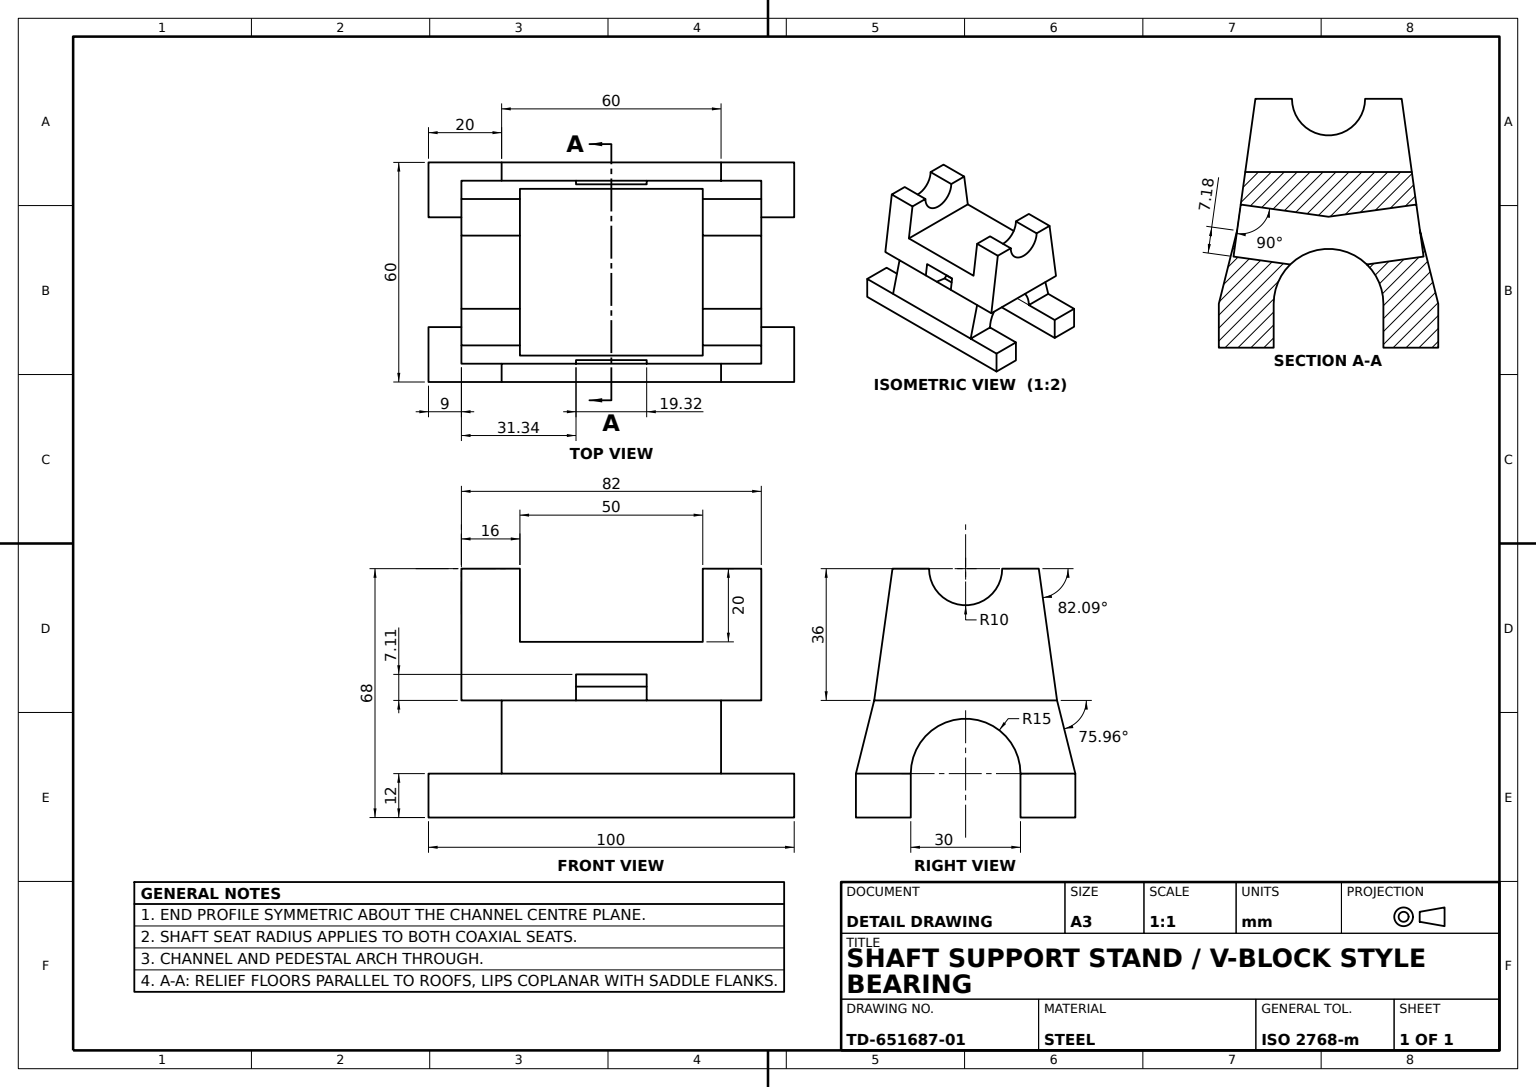
from build123d import *

# Parameters (mm, degrees)
BASE_BLOCK_DEPTH             = 12
BASE_CHANNEL_CUT_30X15_DEPTH = 73
TAPERED_PEDESTAL_DEPTH       = 60
SADDLE_BODY_DEPTH            = 82
SADDLE_RECESS_CUT_DEPTH      = 20
SIDE_RELIEF_SKETCH_W         = 19.32494716
SIDE_RELIEF_SKETCH_H         = 14.354217055
SIDE_RELIEF_CUT_DEPTH        = 28


with BuildPart() as part:
    # Base Profile Sketch → Base Block (new body)
    with BuildSketch(Plane(origin=(0, 0, 0), x_dir=(1, 0, 0), z_dir=(0, 1, 0))):
        Polygon((0, 0), (30, 0), (30, 100), (-30, 100), (-30, 0), align=None)
    extrude(amount=BASE_BLOCK_DEPTH)

    # Base Channel Sketch → Base Channel Cut 30x15 (cut)
    with BuildSketch(Plane(origin=(0, 12, 0), x_dir=(1, 0, 0), z_dir=(0, 1, 0))):
        Polygon((0, 0), (15, 0), (15, 100), (-15, 100), (-15, 0), align=None)
    extrude(amount=-BASE_CHANNEL_CUT_30X15_DEPTH, mode=Mode.SUBTRACT)


with BuildPart() as base_channel_cut_30x15_piece_1:
    # of the separate pieces the step leaves, piece 1, a body of its own (base_channel_cut_30x15_pieces)
    add(part.part.solids().sort_by_distance((30, 0, 0))[0])



with BuildPart() as base_channel_cut_30x15_piece_2:
    # of the separate pieces the step leaves, piece 2, a body of its own (base_channel_cut_30x15_pieces)
    add(part.part.solids().sort_by_distance((-15, 12, 0))[0])


with BuildPart() as base_channel_cut_30x15_piece_1_1:
    add(base_channel_cut_30x15_piece_1.part)

    add(base_channel_cut_30x15_piece_2.part)  # Tapered Pedestal merges Base Channel Cut 30x15 piece 2
    # Pedestal Profile Sketch → Tapered Pedestal (add)
    with BuildSketch(Plane.XY.offset(-20)):
        with BuildLine():
            Line((0, 32), (25, 32))
            Line((25, 32), (30, 12))
            Line((30, 12), (15, 12))
            ThreePointArc((15, 12), (0, 27), (-15, 12))
            Line((-15, 12), (-30, 12))
            Line((-30, 12), (-25, 32))
            Line((-25, 32), (0, 32))
        make_face()
    extrude(amount=-TAPERED_PEDESTAL_DEPTH)

    # Saddle Profile Sketch → Saddle Body (add)
    with BuildSketch(Plane.XY.offset(-9)):
        with BuildLine():
            Line((10, 68), (20, 68))
            Line((20, 68), (25, 32))
            Line((25, 32), (-10.572876043, 32))
            Line((-10.572876043, 32), (-25, 32))
            Line((-25, 32), (-20, 68))
            Line((-20, 68), (-10, 68))
            ThreePointArc((-10, 68), (0, 58), (10, 68))
        make_face()
    extrude(amount=-SADDLE_BODY_DEPTH)

    # Saddle Recess Sketch → Saddle Recess Cut (cut)
    with BuildSketch(Plane(origin=(0, 68, 0), x_dir=(1, 0, 0), z_dir=(0, 1, 0))):
        Polygon((20, 75), (-20, 75), (-29.513236355, 75), (-29.513236355, 25), (-20, 25), (20, 25), (26.893267856, 25), (26.893267856, 75), align=None)
    extrude(amount=-SADDLE_RECESS_CUT_DEPTH, mode=Mode.SUBTRACT)

    # Side Relief Sketch → Side Relief Cut (cut)
    with BuildSketch(Plane(origin=(28.887206662, 4.012112036, 0), x_dir=(0, 0, -1), z_dir=(0.9904922731777517, 0.13756837127468668, 0))):
        with Locations((50, 28.25654346)):
            Rectangle(SIDE_RELIEF_SKETCH_W, SIDE_RELIEF_SKETCH_H)
    side_relief_cut = extrude(amount=-SIDE_RELIEF_CUT_DEPTH, mode=Mode.SUBTRACT)

    # Side Relief Mirror: Side Relief Cut across plane
    add(side_relief_cut.mirror(Plane(origin=(0, 0, 0), x_dir=(0, 0, 1), z_dir=(1, 0, 0))), mode=Mode.SUBTRACT)


solid = base_channel_cut_30x15_piece_1_1.part
